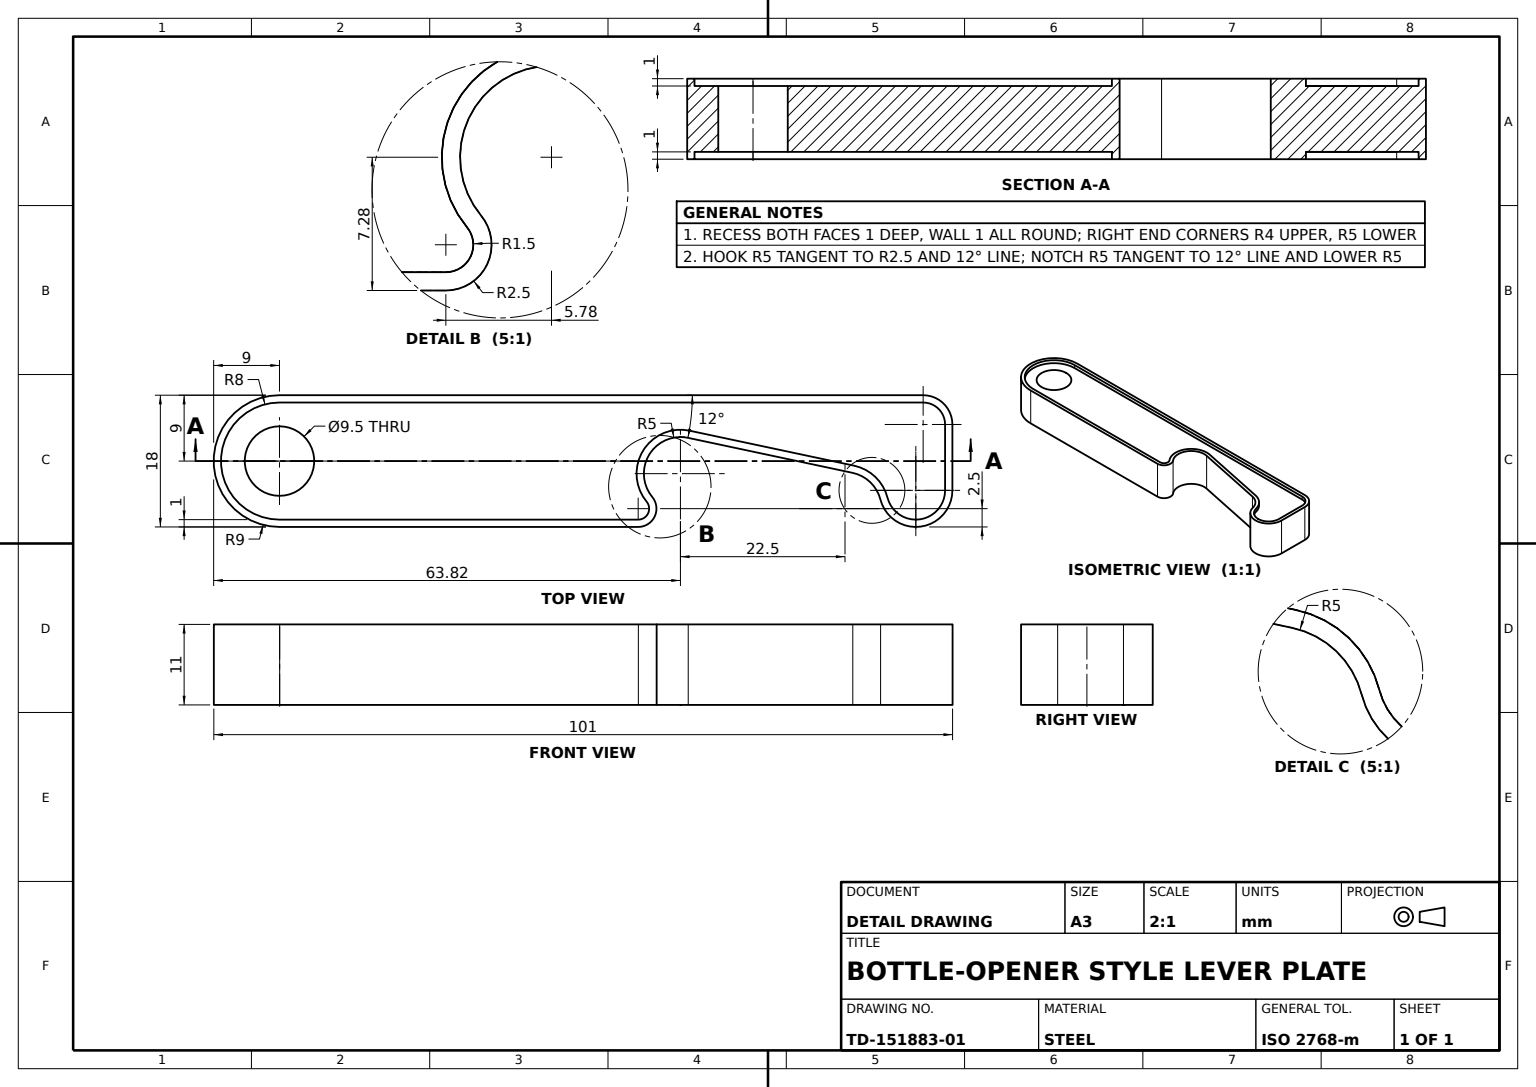
from build123d import *

# Parameters (mm, degrees)
LEVER_PROFILE_SKETCH_R    = 4.75
LEVER_BODY_11MM_DEPTH     = 5.5
TOP_FACE_RECESS_1MM_DEPTH = 1


with BuildPart() as part:
    # Lever Profile Sketch → Lever Body 11mm (new, symmetric)
    with BuildSketch(Plane(origin=(0, 0, 0), x_dir=(1, 0, 0), z_dir=(0, 1, 0))):
        with BuildLine():
            Line((46.5, 9), (-41.5, 9))
            ThreePointArc((-41.5, 9), (-50.5, 0), (-41.5, -9))
            Line((-41.5, -9), (7.540217235, -9))
            ThreePointArc((7.540217235, -9), (9.802454571, -7.564087513), (9.465992035, -4.905825787))
            ThreePointArc((9.465992035, -4.905825787), (9.040307373, 0.871975682), (14.357100089, 3.173260641))
            Line((14.357100089, 3.173260641), (36.857100089, -1.609261996))
            ThreePointArc((36.857100089, -1.609261996), (39.275815642, -2.888858783), (40.658770817, -5.25))
            ThreePointArc((40.658770817, -5.25), (46.130021462, -8.960148481), (50.5, -4))
            Line((50.5, -4), (50.5, 5))
            ThreePointArc((50.5, 5), (49.328427125, 7.828427125), (46.5, 9))
        make_face()
        with Locations(Location((-41.5, 0, 0), (0, 0, 270))):
            Circle(LEVER_PROFILE_SKETCH_R, mode=Mode.SUBTRACT)
    extrude(amount=LEVER_BODY_11MM_DEPTH, both=True)

    # Face Recess Sketch → Top Face Recess 1mm (cut)
    with BuildSketch(Plane(origin=(0, 5.5, 0), x_dir=(1, 0, 0), z_dir=(0, 1, 0))):
        with BuildLine():
            Line((-41.5, -8), (7.540217235, -8))
            ThreePointArc((7.540217235, -8), (8.897559636, -7.138452508), (8.695682115, -5.543495472))
            ThreePointArc((8.695682115, -5.543495472), (8.18486052, 1.389866291), (14.565011779, 4.151408242))
            Line((14.565011779, 4.151408242), (37.065011779, -0.631114396))
            ThreePointArc((37.065011779, -0.631114396), (39.967470443, -2.166630539), (41.627016654, -5))
            ThreePointArc((41.627016654, -5), (46.00401717, -7.968118785), (49.5, -4))
            Line((49.5, -4), (49.5, 5))
            ThreePointArc((49.5, 5), (48.621320344, 7.121320344), (46.5, 8))
            Line((46.5, 8), (-41.5, 8))
            ThreePointArc((-41.5, 8), (-49.5, 0), (-41.5, -8))
        make_face()
    top_face_recess_1mm = extrude(amount=-TOP_FACE_RECESS_1MM_DEPTH, mode=Mode.SUBTRACT)

    # Bottom Face Recess Mirror: Top Face Recess 1mm across plane
    add(top_face_recess_1mm.mirror(Plane.ZX), mode=Mode.SUBTRACT)


solid = part.part
